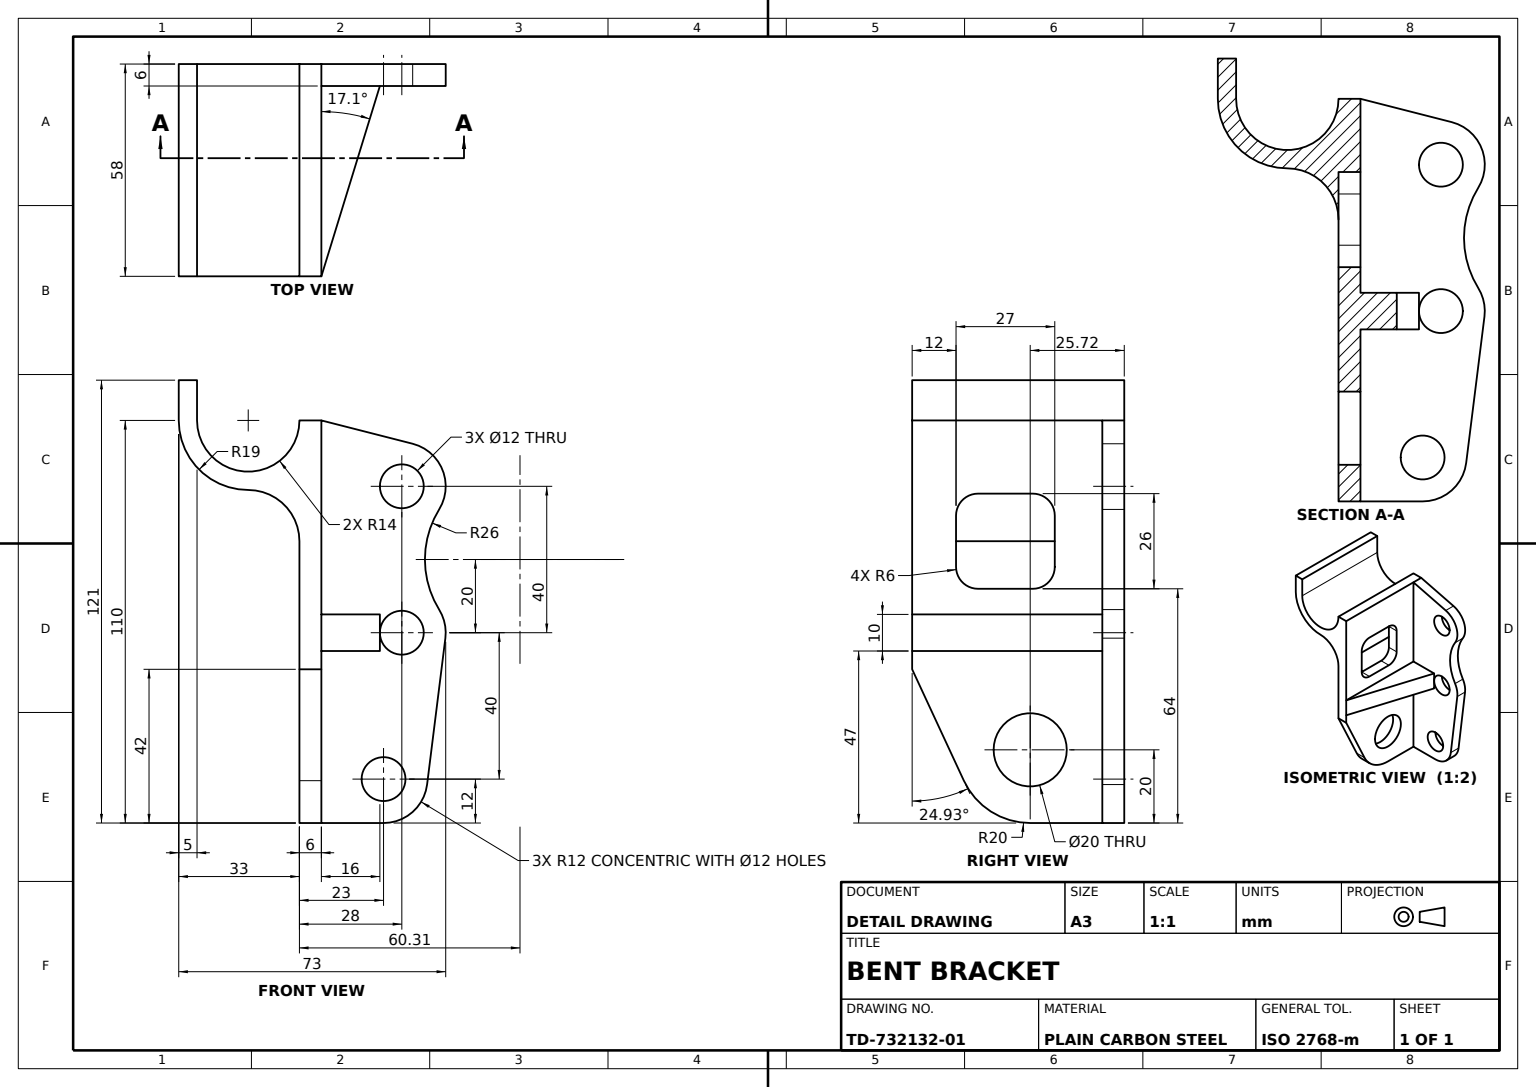
SolidWorks part; units mm, degrees
material "Plain Carbon Steel"
ref_plane "Front Plane" through (0, 0, 0) normal (0, 0, 1) x (1, 0, 0)
ref_plane "Top Plane" through (0, 0, 0) normal (0, 1, 0) x (1, 0, 0)
ref_plane "Right Plane" through (0, 0, 0) normal (1, 0, 0) x (0, 0, -1)
sketch "Back Plate Profile" plane through (0, 0, 0) normal (0, 0, 1) x (1, 0, 0)
  line L1 (0, 0) -> (6, 0)
  line L2 (6, 0) -> (30.9677, -6.3728)
  line L3 (23, -110) -> (0, -110)
  line L4 (0, -110) -> (0, 0)
  line L5 (34.9073, -99.4884) -> (39.9073, -59.4884)
  arc A0 (38.2035, -24.3158) -> (30.9677, -6.3728) centre (28, -18) ccw
  arc A1 (39.9073, -59.4884) -> (38.2035, -51.6842) centre (28, -58) ccw
  arc A2 (23, -110) -> (34.9073, -99.4884) centre (23, -98) ccw
  circle A3 centre (23, -98) radius 6
  arc A4 (38.2035, -51.6842) -> (38.2035, -24.3158) centre (60.311, -38) cw
  circle A5 centre (28, -58) radius 6
  circle A6 centre (28, -18) radius 6
  dimension "D1" = 24
  dimension "D8" = 12
  dimension "D9" = 26
  dimension "D2" = 23
  dimension "D3" = 6
  dimension "D4" = 28
  dimension "D5" = 40
  dimension "D6" = 40
  dimension "D7" = 110
extrude "Back Plate 6mm" add sketch "Back Plate Profile" along normal blind 6
sketch "Side Flange Profile" plane through (0, 0, 0) normal (1, 0, 0) x (0, 0, -1)
  line L0 (0, 0) -> (-58, 0)
  line L1 (-58, 0) -> (-58, -68)
  line L2 (-5.7215, -110) -> (-25.7215, -110)
  line L3 (-58, -68) -> (-43.8586, -98.4289)
  line L4 (-5.7215, -110) -> (0, -110)
  line L5 (-6, -110) -> (0, -110) construction
  line L6 (0, -110) -> (0, 0)
  line L8 (-40, -46) -> (-25, -46)
  line L9 (-46, -40) -> (-46, -26)
  line L10 (-40, -20) -> (-25, -20)
  line L11 (-19, -40) -> (-19, -26)
  line L12 (-46, -46) -> (-19, -20) construction
  line L13 (-46, -20) -> (-19, -46) construction
  arc A0 (-43.8586, -98.4289) -> (-25.7215, -110) centre (-25.7215, -90) ccw
  circle A1 centre (-25.7215, -90) radius 10
  arc A2 (-25, -46) -> (-19, -40) centre (-25, -40) ccw
  arc A3 (-25, -20) -> (-19, -26) centre (-25, -26) cw
  arc A4 (-46, -26) -> (-40, -20) centre (-40, -26) cw
  arc A5 (-40, -46) -> (-46, -40) centre (-40, -40) cw
  point P6 (-32.5, -33)
  dimension "D1" = 20
  dimension "D3" = 20
  dimension "D8" = 6
  dimension "D2" = 20
  dimension "D4" = 12
  dimension "D5" = 27
  dimension "D6" = 26
  dimension "D7" = 20
  dimension "D9" = 68
  dimension "D10" = 58
  dimension "D11" = 25.7215
extrude "Side Flange 6mm" add sketch "Side Flange Profile" along normal blind 6
ref_plane "Gusset Rib Plane" through (0, -58, 0) normal (0, 1, 0) x (1, 0, 0)
sketch "Gusset Rib Path" plane through (0, -58, 0) normal (0, 1, 0) x (1, 0, 0)
  line L0 (6, -58) -> (22, -6)
  line L1 (30.9677, -6) -> (6, -6) construction
  dimension "D1" = 18
rib "Gusset Rib 10mm" sketch "Gusset Rib Path" sketch "Gusset Rib Path" thickness 10 extrusion direction parallel to sketch draft on no parameters "D1"=10
sketch "Cradle Saddle Profile" plane through (0, 0, 58) normal (0, 0, 1) x (1, 0, 0)
  line L0 (-33, 0) -> (-33, 11)
  line L1 (-33, 11) -> (-28, 11)
  line L2 (-28, 11) -> (-28, 0)
  line L4 (0, 0) -> (0, -68) construction
  line L5 (0, 0) -> (0, -33)
  arc A0 (0, 0) -> (-28, 0) centre (-14, 0) cw
  arc A2 (-33, 0) -> (-14, -19) centre (-14, 0) ccw
  arc A4 (-14, -19) -> (0, -33) centre (-14, -33) cw
  dimension "D1" = 14
  dimension "D2" = 19
  dimension "D4" = 14
  dimension "D3" = 11
  dimension "D5" = 33
extrude "Cradle Saddle" add sketch "Cradle Saddle Profile" against normal up to surface (58 mm away) up to face at (34, -58, 0)
